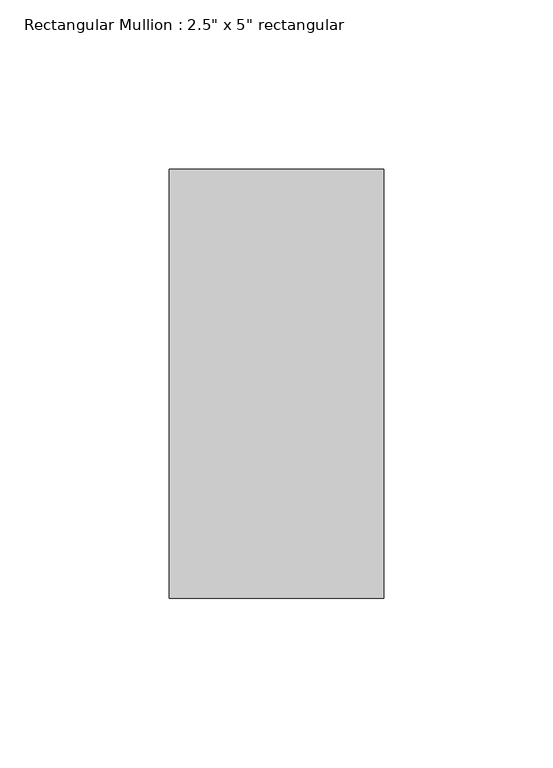
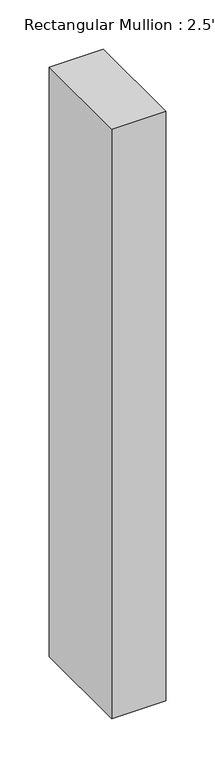
"""IFC4 building model written with IfcOpenShell, lengths in millimetres: member geometry."""

from ifc_helpers import new_model, si_unit, frame, origin, place, context, project, spatial, polyline, outline, extrude, source, transform, mapped, element, save


def member_4a3a2774(model_context):
    return source(origin(), model_context, "Body", "SweptSolid", [
        extrude(outline(polyline([(31.75, 63.5), (31.75, -63.5), (-31.75, -63.5), (-31.75, 63.5), (31.75, 63.5)])), frame((0.0, 0.0, -732.3666667), z_axis=(0.0, 0.0, 1.0), x_axis=(1.0, 0.0, 0.0)), (0.0, 0.0, 1.0), 732.3666667),
    ])


if __name__ == "__main__":
    model = new_model("IFC4")
    model_context = context("Model", 3, world=origin())
    ifc_project = project(units=[si_unit("LENGTHUNIT", "METRE", prefix="MILLI")], contexts=[model_context])
    site = spatial("IfcSite", under=ifc_project)
    building = spatial("IfcBuilding", under=site)
    placement = place(None, origin())
    member_shape = member_4a3a2774(model_context)
    element("IfcMember", 1, ObjectType="Rectangular Mullion : 2.5\" x 5\" rectangular", at=placement, inside=building, context=model_context, shape_type="MappedRepresentation", body=[
        mapped(member_shape, transform((0.0, 0.0, 0.0), x_axis=(1.0, 0.0, 0.0), y_axis=(0.0, 1.0, 0.0), z_axis=(0.0, 0.0, 1.0))),
    ])
    save(model, "model.ifc")

# Revit data of these elements
# Type "Rectangular Mullion : 2.5\" x 5\" rectangular"
#   built-in parameter 1007304 = 0.416667 (stored number, unit not read)
#   built-in parameter 1007301 = 0.104167 (stored number, unit not read)
#   built-in parameter 1007300 = 0.104167 (stored number, unit not read)
# Element 1 (IfcMember, "Rectangular Mullion : 2.5\" x 5\" rectangular")
#   Materials on its faces: "Aluminum"
# Materials
#   "Aluminum": class "Metal", colour RGB 247 247 247, transparency 0, Description = "Aluminum 6061", Cost = 0
